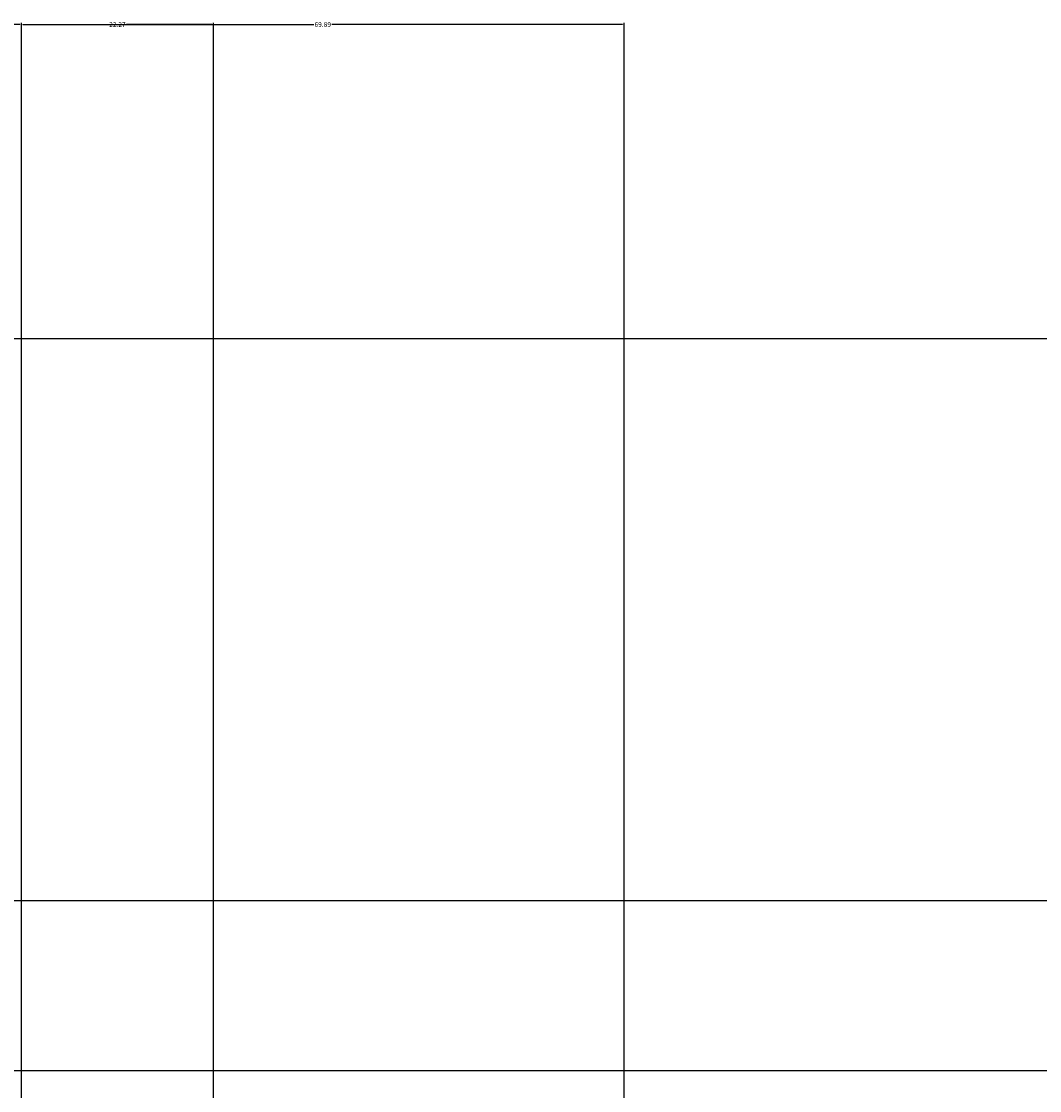
# Model space of a CAD drawing. Units: inches. Extents: x -26 to 776, y -22 to 650.
# Tile 61 of 62: x 426 to 544, y 526 to 650. Entities that reach past the tile are written whole.
import ezdxf

# ---------------------------------------------------------------- set-up
doc = ezdxf.new("R2010")
doc.units = ezdxf.units.IN
doc.header["$MEASUREMENT"] = 0
doc.layers.add('A-ANNO-DIMS', color=2, linetype='Continuous', lineweight=18)
doc.styles.get("Standard").update_dxf_attribs({"font": 'arial.ttf'})
doc.dimstyles.get("Standard").update_dxf_attribs({"dimtxt": 0.5625, "dimasz": 0.18, "dimexe": 0.18, "dimexo": 0.0625, "dimgap": 0.09, "dimtad": 0, "dimtih": 1, "dimtoh": 1, "dimdec": 4, "dimzin": 0, "dimdsep": 46, "dimlunit": 4, "dimtxsty": 'Standard', "dimcen": 0.09, "dimadec": 0, "dimazin": 0, "dimtfac": 1, "dimtdec": 4, "dimtofl": 0, "dimtmove": 0, "dimatfit": 3, "dimfxl": 1, "dimtolj": 1, "dimtzin": 0, "dimarcsym": 0})

# ---------------------------------------------------------------- blocks, each defined once
blk = doc.blocks.new('*D21')
at = {"layer": 'A-ANNO-DIMS', "color": 0, "lineweight": -2, "transparency": 16777216}
for p, q in [((425.74, 455.53), (425.74, 649.86)), ((425.92, 649.68), (435.83, 649.68)), ((447.83, 649.68), (437.92, 649.68)), ((448.01, 444.45), (448.01, 649.86))]:
    blk.add_line(p, q, dxfattribs=at)
at = {"layer": 'A-ANNO-DIMS', "color": 0, "transparency": 16777216}
for points in [[(425.92, 649.71), (425.92, 649.65), (425.74, 649.68)], [(447.83, 649.71), (447.83, 649.65), (448.01, 649.68)]]:
    blk.add_solid(points, dxfattribs=at)
at = {"layer": 'Defpoints', "color": 0, "transparency": 16777216}
for p in [(448.01, 649.68), (425.74, 455.47), (448.01, 444.39)]:
    blk.add_point(p, dxfattribs=at)
at = {"layer": 'A-ANNO-DIMS', "color": 0, "transparency": 16777216, "insert": (436.88, 649.68), "char_height": 0.562, "attachment_point": 5}
blk.add_mtext('\\A1;22.27', dxfattribs=at)
blk = doc.blocks.new('*D32')
at = {"layer": 'A-ANNO-DIMS', "color": 0, "lineweight": -2, "transparency": 16777216}
for p, q in [((357.13, 613.27), (775.34, 613.27)), ((775.16, 613.09), (775.16, 581.06)), ((775.16, 548.28), (775.16, 580.31)), ((357.37, 548.1), (775.34, 548.1))]:
    blk.add_line(p, q, dxfattribs=at)
at = {"layer": 'A-ANNO-DIMS', "color": 0, "transparency": 16777216}
for points in [[(775.13, 613.09), (775.19, 613.09), (775.16, 613.27)], [(775.13, 548.28), (775.19, 548.28), (775.16, 548.1)]]:
    blk.add_solid(points, dxfattribs=at)
at = {"layer": 'Defpoints', "color": 0, "transparency": 16777216}
for p in [(357.07, 613.27), (775.16, 613.27), (357.3, 548.1)]:
    blk.add_point(p, dxfattribs=at)
at = {"layer": 'A-ANNO-DIMS', "color": 0, "transparency": 16777216, "insert": (775.16, 580.69), "char_height": 0.562, "attachment_point": 5}
blk.add_mtext('\\A1;65.17', dxfattribs=at)
blk = doc.blocks.new('*D33')
at = {"layer": 'A-ANNO-DIMS', "color": 0, "lineweight": -2, "transparency": 16777216}
for p, q in [((357.37, 548.1), (775.34, 548.1)), ((775.16, 547.92), (775.16, 538.64)), ((775.16, 528.6), (775.16, 537.88)), ((357.37, 528.42), (775.34, 528.42))]:
    blk.add_line(p, q, dxfattribs=at)
at = {"layer": 'A-ANNO-DIMS', "color": 0, "transparency": 16777216}
for points in [[(775.13, 547.92), (775.19, 547.92), (775.16, 548.1)], [(775.13, 528.6), (775.19, 528.6), (775.16, 528.42)]]:
    blk.add_solid(points, dxfattribs=at)
at = {"layer": 'Defpoints', "color": 0, "transparency": 16777216}
for p in [(357.3, 548.1), (775.16, 548.1), (357.3, 528.42)]:
    blk.add_point(p, dxfattribs=at)
at = {"layer": 'A-ANNO-DIMS', "color": 0, "transparency": 16777216, "insert": (775.16, 538.26), "char_height": 0.562, "attachment_point": 5}
blk.add_mtext('\\A1;19.676', dxfattribs=at)
blk = doc.blocks.new('*D39')
at = {"layer": 'A-ANNO-DIMS', "color": 0, "lineweight": -2, "transparency": 16777216}
for p, q in [((289.24, 15.54), (289.24, 649.86)), ((289.42, 649.68), (356.48, 649.68)), ((425.56, 649.68), (358.51, 649.68)), ((425.74, 15.54), (425.74, 649.86))]:
    blk.add_line(p, q, dxfattribs=at)
at = {"layer": 'A-ANNO-DIMS', "color": 0, "transparency": 16777216}
for points in [[(289.42, 649.71), (289.42, 649.65), (289.24, 649.68)], [(425.56, 649.71), (425.56, 649.65), (425.74, 649.68)]]:
    blk.add_solid(points, dxfattribs=at)
at = {"layer": 'Defpoints', "color": 0, "transparency": 16777216}
for p in [(425.74, 649.68), (289.24, 15.48), (425.74, 15.48)]:
    blk.add_point(p, dxfattribs=at)
at = {"layer": 'A-ANNO-DIMS', "color": 0, "transparency": 16777216, "insert": (357.49, 649.68), "char_height": 0.562, "attachment_point": 5}
blk.add_mtext('\\A1;136.5', dxfattribs=at)
blk = doc.blocks.new('*D40')
at = {"layer": 'A-ANNO-DIMS', "color": 0, "lineweight": -2, "transparency": 16777216}
for p, q in [((425.74, 15.54), (425.74, 649.86)), ((425.92, 649.68), (459.65, 649.68)), ((495.45, 649.68), (461.73, 649.68)), ((495.63, 15.54), (495.63, 649.86))]:
    blk.add_line(p, q, dxfattribs=at)
at = {"layer": 'A-ANNO-DIMS', "color": 0, "transparency": 16777216}
for points in [[(425.92, 649.71), (425.92, 649.65), (425.74, 649.68)], [(495.45, 649.71), (495.45, 649.65), (495.63, 649.68)]]:
    blk.add_solid(points, dxfattribs=at)
at = {"layer": 'Defpoints', "color": 0, "transparency": 16777216}
for p in [(495.63, 649.68), (425.74, 15.48), (495.63, 15.48)]:
    blk.add_point(p, dxfattribs=at)
at = {"layer": 'A-ANNO-DIMS', "color": 0, "transparency": 16777216, "insert": (460.69, 649.68), "char_height": 0.562, "attachment_point": 5}
blk.add_mtext('\\A1;69.89', dxfattribs=at)

msp = doc.modelspace()

# ---------------------------------------------------------------- dimensions: what is measured, and where the dimension line sits
at = {"layer": 'A-ANNO-DIMS'}
for base, p1, p2, override, picture, middle in [((425.7434, 649.6763), (289.2424, 15.4824), (425.7434, 15.4824), {"dimdec": 1, "dimlfac": 1, "dimrnd": 0, "dimzin": 0, "dimdsep": 46, "dimlunit": 2}, '*D39', (357.4929, 649.6763)), ((448.0125, 649.6763), (425.7434, 455.4717), (448.0125, 444.3909), {"dimdec": 2, "dimlfac": 1, "dimrnd": 0, "dimzin": 0, "dimdsep": 46, "dimlunit": 2}, '*D21', (436.878, 649.6763)), ((495.6309, 649.6763), (425.7434, 15.4824), (495.6309, 15.4824), {"dimdec": 2, "dimlfac": 1, "dimrnd": 0, "dimzin": 0, "dimdsep": 46, "dimlunit": 2}, '*D40', (460.6872, 649.6763))]:
    dim = msp.add_linear_dim(base=base, p1=p1, p2=p2, dimstyle='Standard', override=override, dxfattribs=at)
    dim.commit()
    dim.dimension.update_dxf_attribs({"geometry": picture, "text_midpoint": middle})
for base, p1, p2, override, picture, middle in [((775.1553, 613.2713), (357.3034, 548.0996), (357.0669, 613.2713), {"dimdec": 2, "dimlfac": 1, "dimrnd": 0, "dimzin": 0, "dimdsep": 46, "dimlunit": 2}, '*D32', (775.1553, 580.6855)), ((775.1553, 548.0996), (357.3034, 528.4233), (357.3034, 548.0996), {"dimdec": 3, "dimlfac": 1, "dimrnd": 0, "dimzin": 0, "dimdsep": 46, "dimlunit": 2}, '*D33', (775.1553, 538.2614))]:
    dim = msp.add_linear_dim(base=base, p1=p1, p2=p2, angle=90, dimstyle='Standard', override=override, dxfattribs=at)
    dim.commit()
    dim.dimension.update_dxf_attribs({"geometry": picture, "text_midpoint": middle})

doc.saveas('drawing.dxf')
